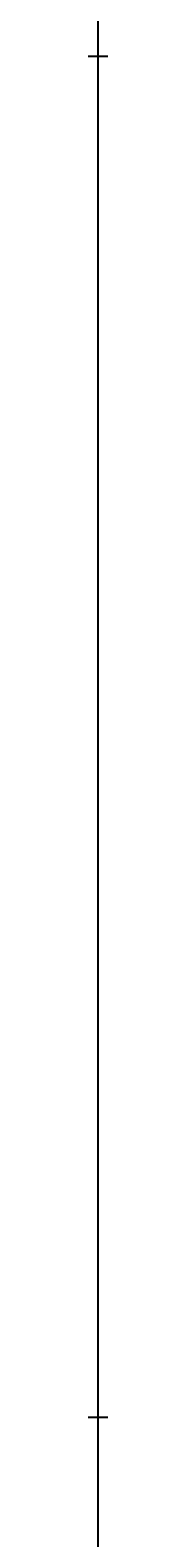
# Model space of a CAD drawing. Units: inches. Extents: x 35362 to 73946, y 43607 to 67532.
# Tile 35 of 134: x 48373 to 48373, y 46091 to 46564. Entities that reach past the tile are written whole.
import ezdxf

# ---------------------------------------------------------------- set-up
doc = ezdxf.new("R2010")
doc.units = ezdxf.units.IN
doc.header["$MEASUREMENT"] = 0
doc.layers.add('A-ANNO-DIMS', color=2, linetype='Continuous', lineweight=18)
doc.styles.get("Standard").update_dxf_attribs({"font": 'arial.ttf'})
doc.dimstyles.get("Standard").update_dxf_attribs({"dimtxt": 0.18, "dimasz": 0.18, "dimexe": 0.18, "dimexo": 0.0625, "dimgap": 0.09, "dimtad": 0, "dimtih": 1, "dimtoh": 1, "dimdec": 4, "dimzin": 0, "dimdsep": 46, "dimtxsty": 'Standard', "dimcen": 0.09, "dimadec": 0, "dimazin": 0, "dimtfac": 1, "dimtdec": 4, "dimtofl": 0, "dimtmove": 0, "dimatfit": 3, "dimfxl": 1, "dimtolj": 1, "dimtzin": 0, "dimarcsym": 0})

# ---------------------------------------------------------------- blocks, each defined once
blk = doc.blocks.new('*D5')
at = {"layer": 'A-ANNO-DIMS', "color": 0, "lineweight": -2, "transparency": 16777216}
for p, q in [((37121.95, 46919.32), (37121.95, 43606.68)), ((69871.5, 45449.83), (69871.5, 43606.68)), ((37122.13, 43606.86), (53496.29, 43606.86)), ((69871.32, 43606.86), (53497.15, 43606.86))]:
    blk.add_line(p, q, dxfattribs=at)
at = {"layer": 'A-ANNO-DIMS', "color": 0, "transparency": 16777216}
for points in [[(37122.13, 43606.89), (37122.13, 43606.83), (37121.95, 43606.86)], [(69871.32, 43606.89), (69871.32, 43606.83), (69871.5, 43606.86)]]:
    blk.add_solid(points, dxfattribs=at)
at = {"layer": 'Defpoints', "color": 0, "transparency": 16777216}
for p in [(37121.95, 46919.38), (69871.5, 45449.89), (69871.5, 43606.86)]:
    blk.add_point(p, dxfattribs=at)
at = {"layer": 'A-ANNO-DIMS', "color": 0, "transparency": 16777216, "insert": (53496.72, 43606.86), "char_height": 0.18, "attachment_point": 5}
blk.add_mtext('\\A1;32750', dxfattribs=at)
blk = doc.blocks.new('*D11')
at = {"layer": 'A-ANNO-DIMS', "color": 0, "lineweight": -2, "transparency": 16777216}
for p, q in [((47978.66, 56028.77), (47978.66, 43606.68)), ((53109.76, 56028.77), (53109.76, 43606.68)), ((47978.84, 43606.86), (50543.87, 43606.86)), ((53109.58, 43606.86), (50544.55, 43606.86))]:
    blk.add_line(p, q, dxfattribs=at)
at = {"layer": 'A-ANNO-DIMS', "color": 0, "transparency": 16777216}
for points in [[(47978.84, 43606.89), (47978.84, 43606.83), (47978.66, 43606.86)], [(53109.58, 43606.89), (53109.58, 43606.83), (53109.76, 43606.86)]]:
    blk.add_solid(points, dxfattribs=at)
at = {"layer": 'Defpoints', "color": 0, "transparency": 16777216}
for p in [(47978.66, 56028.84), (53109.76, 56028.84), (53109.76, 43606.86)]:
    blk.add_point(p, dxfattribs=at)
at = {"layer": 'A-ANNO-DIMS', "color": 0, "transparency": 16777216, "insert": (50544.21, 43606.86), "char_height": 0.18, "attachment_point": 5}
blk.add_mtext('\\A1;5131', dxfattribs=at)
blk = doc.blocks.new('*D13')
at = {"layer": 'A-ANNO-DIMS', "color": 0, "lineweight": -2, "transparency": 16777216}
for p, q in [((48373.49, 51694.02), (48373.49, 43606.68)), ((51029.04, 51694.02), (51029.04, 43606.68)), ((48373.67, 43606.86), (49700.8, 43606.86)), ((51028.86, 43606.86), (49701.73, 43606.86))]:
    blk.add_line(p, q, dxfattribs=at)
at = {"layer": 'A-ANNO-DIMS', "color": 0, "transparency": 16777216}
for points in [[(48373.67, 43606.89), (48373.67, 43606.83), (48373.49, 43606.86)], [(51028.86, 43606.89), (51028.86, 43606.83), (51029.04, 43606.86)]]:
    blk.add_solid(points, dxfattribs=at)
at = {"layer": 'Defpoints', "color": 0, "transparency": 16777216}
for p in [(48373.49, 51694.09), (51029.04, 51694.09), (51029.04, 43606.86)]:
    blk.add_point(p, dxfattribs=at)
at = {"layer": 'A-ANNO-DIMS', "color": 0, "transparency": 16777216, "insert": (49701.27, 43606.86), "char_height": 0.18, "attachment_point": 5}
blk.add_mtext('\\A1;2655.6', dxfattribs=at)
blk = doc.blocks.new('*D67')
at = {"layer": 'A-ANNO-DIMS', "color": 0, "lineweight": -2, "transparency": 16777216}
for p, q in [((56873.54, 53351.53), (35361.77, 53351.53)), ((35361.95, 53351.35), (35361.95, 49400.89)), ((35361.95, 45450.07), (35361.95, 49400.53)), ((53793.58, 45449.89), (35361.77, 45449.89))]:
    blk.add_line(p, q, dxfattribs=at)
at = {"layer": 'A-ANNO-DIMS', "color": 0, "transparency": 16777216}
for points in [[(35361.92, 53351.35), (35361.98, 53351.35), (35361.95, 53351.53)], [(35361.92, 45450.07), (35361.98, 45450.07), (35361.95, 45449.89)]]:
    blk.add_solid(points, dxfattribs=at)
at = {"layer": 'Defpoints', "color": 0, "transparency": 16777216}
for p in [(35361.95, 53351.53), (56873.6, 53351.53), (53793.64, 45449.89)]:
    blk.add_point(p, dxfattribs=at)
at = {"layer": 'A-ANNO-DIMS', "color": 0, "transparency": 16777216, "insert": (35361.95, 49400.71), "char_height": 0.18, "attachment_point": 5}
blk.add_mtext('\\A1;7901.6', dxfattribs=at)
blk = doc.blocks.new('*D76')
at = {"layer": 'A-ANNO-DIMS', "color": 0, "lineweight": -2, "transparency": 16777216}
for p, q in [((54052.84, 46555.29), (35361.77, 46555.29)), ((35361.95, 46555.11), (35361.95, 46342.27)), ((35361.95, 46129.06), (35361.95, 46341.9)), ((53793.58, 46128.88), (35361.77, 46128.88))]:
    blk.add_line(p, q, dxfattribs=at)
at = {"layer": 'A-ANNO-DIMS', "color": 0, "transparency": 16777216}
for points in [[(35361.92, 46555.11), (35361.98, 46555.11), (35361.95, 46555.29)], [(35361.92, 46129.06), (35361.98, 46129.06), (35361.95, 46128.88)]]:
    blk.add_solid(points, dxfattribs=at)
at = {"layer": 'Defpoints', "color": 0, "transparency": 16777216}
for p in [(35361.95, 46555.29), (54052.9, 46555.29), (53793.64, 46128.88)]:
    blk.add_point(p, dxfattribs=at)
at = {"layer": 'A-ANNO-DIMS', "color": 0, "transparency": 16777216, "insert": (35361.95, 46342.09), "char_height": 0.18, "attachment_point": 5}
blk.add_mtext('\\A1;426.4', dxfattribs=at)
blk = doc.blocks.new('*D90')
at = {"layer": 'A-ANNO-DIMS', "color": 0, "lineweight": -2, "transparency": 16777216}
for p, q in [((53707.72, 47291.29), (35361.77, 47291.29)), ((35361.95, 47291.11), (35361.95, 46710.26)), ((35361.95, 46129.06), (35361.95, 46709.9)), ((53793.58, 46128.88), (35361.77, 46128.88))]:
    blk.add_line(p, q, dxfattribs=at)
at = {"layer": 'A-ANNO-DIMS', "color": 0, "transparency": 16777216}
for points in [[(35361.92, 47291.11), (35361.98, 47291.11), (35361.95, 47291.29)], [(35361.92, 46129.06), (35361.98, 46129.06), (35361.95, 46128.88)]]:
    blk.add_solid(points, dxfattribs=at)
at = {"layer": 'Defpoints', "color": 0, "transparency": 16777216}
for p in [(53707.78, 47291.29), (35361.95, 46128.88), (53793.64, 46128.88)]:
    blk.add_point(p, dxfattribs=at)
at = {"layer": 'A-ANNO-DIMS', "color": 0, "transparency": 16777216, "insert": (35361.95, 46710.08), "char_height": 0.18, "attachment_point": 5}
blk.add_mtext('\\A1;1162.4', dxfattribs=at)

msp = doc.modelspace()

# ---------------------------------------------------------------- dimensions: what is measured, and where the dimension line sits
at = {"layer": 'A-ANNO-DIMS'}
for base, p1, p2, override, picture, middle in [((53109.76, 43606.859), (47978.665, 56028.836), (53109.76, 56028.836), {"dimdec": 0, "dimlfac": 1, "dimrnd": 0, "dimzin": 0, "dimdsep": 46, "dimlunit": 2}, '*D11', (50544.212, 43606.859)), ((51029.043, 43606.859), (48373.492, 51694.087), (51029.043, 51694.087), {"dimdec": 1, "dimlfac": 1, "dimrnd": 0, "dimzin": 0, "dimdsep": 46, "dimlunit": 2}, '*D13', (49701.267, 43606.859)), ((69871.496, 43606.859), (37121.949, 46919.381), (69871.496, 45449.894), {"dimdec": 0, "dimlfac": 1, "dimrnd": 0, "dimzin": 0, "dimdsep": 46, "dimlunit": 2}, '*D5', (53496.723, 43606.859))]:
    dim = msp.add_linear_dim(base=base, p1=p1, p2=p2, dimstyle='Standard', override=override, dxfattribs=at)
    dim.commit()
    dim.dimension.update_dxf_attribs({"geometry": picture, "text_midpoint": middle})
for base, p1, p2, picture, middle in [((35361.949, 53351.529), (53793.638, 45449.894), (56873.602, 53351.529), '*D67', (35361.949, 49400.712)), ((35361.949, 46128.878), (53707.781, 47291.285), (53793.638, 46128.878), '*D90', (35361.949, 46710.081)), ((35361.949, 46555.293), (53793.638, 46128.878), (54052.899, 46555.293), '*D76', (35361.949, 46342.086))]:
    dim = msp.add_linear_dim(base=base, p1=p1, p2=p2, angle=90, dimstyle='Standard', override={"dimdec": 1, "dimlfac": 1, "dimrnd": 0, "dimzin": 0, "dimdsep": 46, "dimlunit": 2}, dxfattribs=at)
    dim.commit()
    dim.dimension.update_dxf_attribs({"geometry": picture, "text_midpoint": middle})

doc.saveas('drawing.dxf')
